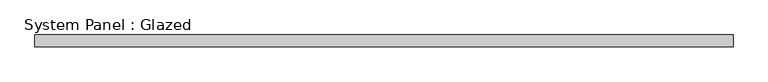
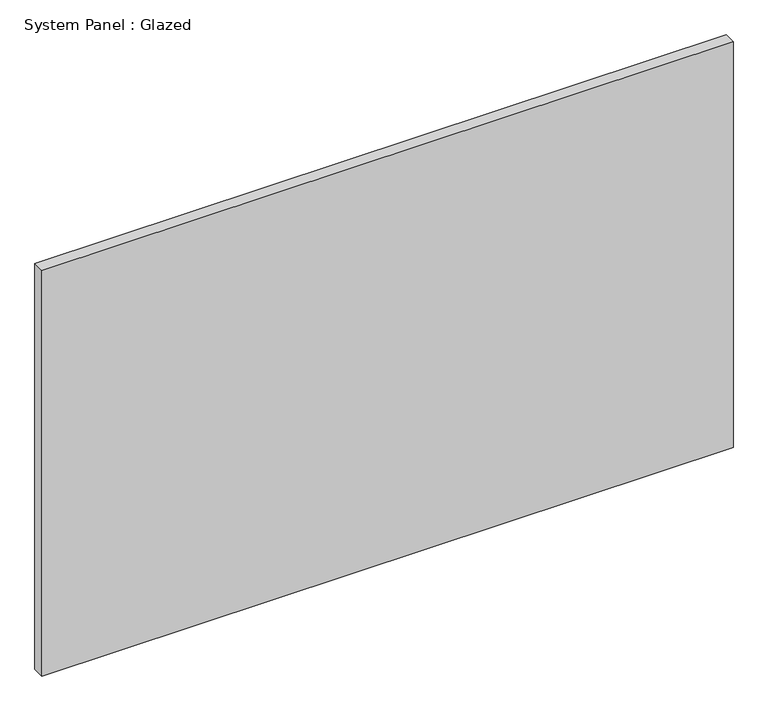
"""IFC4 building model written with IfcOpenShell, lengths in millimetres: plate geometry, System Panel : Glazed."""

from ifc_helpers import new_model, si_unit, origin, origin_with_axes, place, context, project, spatial, polyline, outline, extrude, source, transform, mapped, element, save


def system_panel_glazed_1e00a1c5(model_context):
    return source(origin(), model_context, "Body", "SweptSolid", [
        extrude(outline(polyline([(736.6, 19.05), (-736.6, 19.05), (-736.6, 44.45), (736.6, 44.45), (736.6, 19.05)])), origin_with_axes(), (0.0, 0.0, 1.0), 914.4),
    ])


if __name__ == "__main__":
    model = new_model("IFC4")
    model_context = context("Model", 3, world=origin())
    ifc_project = project(units=[si_unit("LENGTHUNIT", "METRE", prefix="MILLI")], contexts=[model_context])
    site = spatial("IfcSite", under=ifc_project)
    building = spatial("IfcBuilding", under=site)
    placement = place(None, origin())
    system_panel_glazed_shape = system_panel_glazed_1e00a1c5(model_context)
    element("IfcPlate", 1, ObjectType="System Panel : Glazed", at=placement, inside=building, context=model_context, shape_type="MappedRepresentation", body=[
        mapped(system_panel_glazed_shape, transform((0.0, 0.0, 0.0), x_axis=(1.0, 0.0, 0.0), y_axis=(0.0, 1.0, 0.0), z_axis=(0.0, 0.0, 1.0))),
    ])
    save(model, "model.ifc")

# Revit data of these elements
# Type "System Panel : Glazed"
#   Construction Type Id = "GSP4R"
#   Analytic Construction = "1/8 in Pilkington single glazing"
#   Visual Light Transmittance = 0.9
#   Solar Heat Gain Coefficient = 0.86
#   Heat Transfer Coefficient (U) = 6.7069 W/(m²·K)
# Element 1 (IfcPlate, "System Panel : Glazed")
#   Materials on its faces: "Glass"
# Materials
#   "Glass": class "Glass", colour RGB 0 128 192, transparency 0.75, Description = "Soda Lime Glass", Cost = 0
